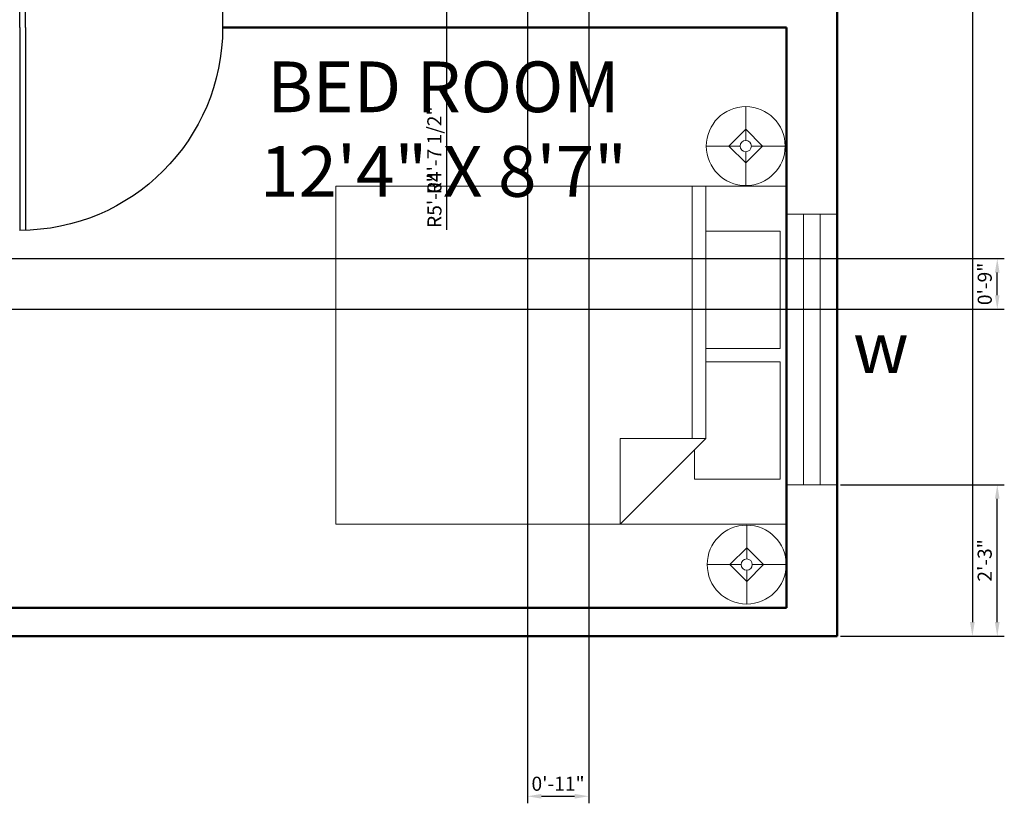
# Model space of a CAD drawing. Units: inches. Extents: x 1962 to 2423, y 2693 to 3296.
# Tile 2 of 4: x 2212 to 2386, y 2694 to 2833. Entities that reach past the tile are written whole.
import ezdxf

# ---------------------------------------------------------------- set-up
doc = ezdxf.new("R2010")
doc.units = ezdxf.units.IN
for name, color, linetype, lineweight in [('A-ANNO-DIMS', 2, 'Continuous', 18), ('A-ANNO-TEXT', 3, 'Continuous', 18), ('A-AREA-IDEN', 7, 'Continuous', 25), ('A-DOOR', 3, 'Continuous', 25), ('A-FURN', 8, 'Continuous', 18), ('A-GLAZ', 4, 'Continuous', 18), ('A-WALL', 7, 'Continuous', 50)]:
    doc.layers.add(name, color=color, linetype=linetype, lineweight=lineweight)
doc.styles.get("Standard").update_dxf_attribs({"font": 'arial.ttf'})
doc.dimstyles.new('ISO-25', dxfattribs={"dimtxt": 2.5, "dimasz": 2.5, "dimexe": 1.25, "dimexo": 0.625, "dimtad": 1, "dimdec": 0, "dimlunit": 3, "dimtxsty": 'Standard', "dimcen": 2.5, "dimadec": 0, "dimazin": 0, "dimtfac": 1, "dimtdec": 0, "dimtmove": 0, "dimatfit": 3, "dimfxl": 1, "dimarcsym": 0})

# ---------------------------------------------------------------- blocks, each defined once
blk = doc.blocks.new('*D13')
at = {"layer": 'A-ANNO-DIMS', "color": 0, "lineweight": -2, "transparency": 16777216}
for p, q in [((2357.16, 3263.59), (2381.77, 3263.59)), ((2380.52, 3261.09), (2380.52, 2726.09)), ((2357.16, 2723.59), (2381.77, 2723.59))]:
    blk.add_line(p, q, dxfattribs=at)
at = {"layer": 'A-ANNO-DIMS', "color": 0, "transparency": 16777216}
for points in [[(2380.1, 3261.09), (2380.94, 3261.09), (2380.52, 3263.59)], [(2380.1, 2726.09), (2380.94, 2726.09), (2380.52, 2723.59)]]:
    blk.add_solid(points, dxfattribs=at)
at = {"layer": 'Defpoints', "color": 0, "transparency": 16777216}
for p in [(2356.54, 3263.59), (2356.54, 2723.59), (2380.52, 2723.59)]:
    blk.add_point(p, dxfattribs=at)
at = {"layer": 'A-ANNO-DIMS', "color": 0, "transparency": 16777216, "insert": (2378.62, 2993.59), "char_height": 2.5, "attachment_point": 5, "rotation": 90}
blk.add_mtext("45'", dxfattribs=at)
blk = doc.blocks.new('Bed - Queen')
for p, q in [((0, -80.00003), (0, 0)), ((0, 0), (59.99999, 0)), ((59.99999, 0), (59.99999, -80.00003)), ((7.99999, -1.2), (28.79998, -1.2)), ((7.99999, -14.4), (7.99999, -1.2)), ((28.79998, -1.2), (28.79998, -14.4)), ((31.19999, -1.2), (51.99999, -1.2)), ((31.19999, -14.4), (31.19999, -1.2)), ((51.99999, -1.2), (51.99999, -16.4)), ((0, -14.4), (44.8, -14.4)), ((59.99999, -29.6), (44.8, -14.4)), ((44.8, -14.4), (44.8, -29.6)), ((44.8, -16.8), (0, -16.8)), ((51.99999, -16.4), (46.79936, -16.4)), ((44.8, -29.6), (59.99999, -29.6)), ((59.99999, -80.00003), (0, -80.00003))]:
    blk.add_line(p, q)
blk = doc.blocks.new('Lamp - Table')
for p, q in [((0, 7), (0, 1)), ((0, 3), (-3, 0)), ((3, 0), (0, 3)), ((-1, 0), (-7, 0)), ((-3, 0), (0, -3)), ((0, -3), (3, 0)), ((1, 0), (7, 0)), ((0, -1), (0, -7))]:
    blk.add_line(p, q)
for radius in [7, 1]:
    blk.add_circle((0, 0), radius)
blk = doc.blocks.new('DOOR-SWING-36IN')
for p, q in [((0, 5), (0, 41)), ((1, 5), (1, 41)), ((0, 5), (0, 0)), ((1, 5), (1, 0)), ((36, 0), (36, 5))]:
    blk.add_line(p, q)
blk.add_arc((0, 5), 36, 0, 90)
blk = doc.blocks.new('WINDOW-48IN')
for p, q in [((0, 48), (0, 0)), ((9, 48), (0, 48)), ((3, 48), (3, 0)), ((6, 0), (6, 48)), ((9, 0), (9, 48)), ((0, 0), (9, 0))]:
    blk.add_line(p, q)
blk = doc.blocks.new('*D62')
at = {"layer": 'A-ANNO-DIMS', "color": 0, "lineweight": -2, "transparency": 16777216}
for p, q in [((2357.16, 2750.46), (2386.19, 2750.46)), ((2384.94, 2726.09), (2384.94, 2747.96)), ((2357.16, 2723.59), (2386.19, 2723.59))]:
    blk.add_line(p, q, dxfattribs=at)
at = {"layer": 'A-ANNO-DIMS', "color": 0, "transparency": 16777216}
for points in [[(2384.52, 2747.96), (2385.35, 2747.96), (2384.94, 2750.46)], [(2384.52, 2726.09), (2385.35, 2726.09), (2384.94, 2723.59)]]:
    blk.add_solid(points, dxfattribs=at)
at = {"layer": 'Defpoints', "color": 0, "transparency": 16777216}
for p in [(2356.54, 2750.46), (2384.94, 2750.46), (2356.54, 2723.59)]:
    blk.add_point(p, dxfattribs=at)
at = {"layer": 'A-ANNO-DIMS', "color": 0, "transparency": 16777216, "insert": (2383.03, 2737.03), "char_height": 2.5, "attachment_point": 5, "rotation": 90}
blk.add_mtext('2\'-3"', dxfattribs=at)
blk = doc.blocks.new('*D65')
at = {"layer": 'A-ANNO-DIMS', "color": 0, "lineweight": -2, "transparency": 16777216}
for p, q in [((2301.59, 2881.95), (2301.59, 2693.94)), ((2312.47, 2879.27), (2312.47, 2693.94)), ((2304.09, 2695.19), (2309.97, 2695.19))]:
    blk.add_line(p, q, dxfattribs=at)
at = {"layer": 'A-ANNO-DIMS', "color": 0, "transparency": 16777216}
for points in [[(2304.09, 2695.61), (2304.09, 2694.77), (2301.59, 2695.19)], [(2309.97, 2695.61), (2309.97, 2694.77), (2312.47, 2695.19)]]:
    blk.add_solid(points, dxfattribs=at)
at = {"layer": 'Defpoints', "color": 0, "transparency": 16777216}
for p in [(2301.59, 2882.58), (2312.47, 2879.9), (2312.47, 2695.19)]:
    blk.add_point(p, dxfattribs=at)
at = {"layer": 'A-ANNO-DIMS', "color": 0, "transparency": 16777216, "insert": (2307.03, 2697.09), "char_height": 2.5, "attachment_point": 5}
blk.add_mtext('0\'-11"', dxfattribs=at)
blk = doc.blocks.new('*D69')
at = {"layer": 'A-ANNO-DIMS', "color": 0, "lineweight": -2, "transparency": 16777216}
for p, q in [((2042.16, 2790.59), (2386.19, 2790.59)), ((2384.94, 2784.09), (2384.94, 2788.09)), ((2042.16, 2781.59), (2386.19, 2781.59))]:
    blk.add_line(p, q, dxfattribs=at)
at = {"layer": 'A-ANNO-DIMS', "color": 0, "transparency": 16777216}
for points in [[(2384.52, 2788.09), (2385.35, 2788.09), (2384.94, 2790.59)], [(2384.52, 2784.09), (2385.35, 2784.09), (2384.94, 2781.59)]]:
    blk.add_solid(points, dxfattribs=at)
at = {"layer": 'Defpoints', "color": 0, "transparency": 16777216}
for p in [(2041.54, 2790.59), (2384.94, 2790.59), (2041.54, 2781.59)]:
    blk.add_point(p, dxfattribs=at)
at = {"layer": 'A-ANNO-DIMS', "color": 0, "transparency": 16777216, "insert": (2383.04, 2786.09), "char_height": 2.5, "attachment_point": 5, "rotation": 90}
blk.add_mtext('0\'-9"', dxfattribs=at)
blk = doc.blocks.new('*D74')
at = {"layer": 'A-ANNO-DIMS', "color": 0, "lineweight": -2, "transparency": 16777216}
for p, q in [((2287.33, 2897.26), (2287.33, 2837.01)), ((2287.33, 2795.71), (2287.33, 2834.51))]:
    blk.add_line(p, q, dxfattribs=at)
at = {"layer": 'A-ANNO-DIMS', "color": 0, "transparency": 16777216}
blk.add_solid([(2286.91, 2834.51), (2287.74, 2834.51), (2287.33, 2837.01)], dxfattribs=at)
at = {"layer": 'Defpoints', "color": 0, "transparency": 16777216}
for p in [(2287.33, 2897.26), (2287.33, 2837.01)]:
    blk.add_point(p, dxfattribs=at)
at = {"layer": 'A-ANNO-DIMS', "color": 0, "transparency": 16777216, "insert": (2285.43, 2800.86), "char_height": 2.5, "attachment_point": 5, "rotation": 89.9997}
blk.add_mtext('R5\'-0"', dxfattribs=at)
blk = doc.blocks.new('*D75')
at = {"layer": 'A-ANNO-DIMS', "color": 0, "lineweight": -2, "transparency": 16777216}
for p, q in [((2287.33, 2898.39), (2287.33, 2843.01)), ((2287.33, 2801.72), (2287.33, 2840.51))]:
    blk.add_line(p, q, dxfattribs=at)
at = {"layer": 'A-ANNO-DIMS', "color": 0, "transparency": 16777216}
blk.add_solid([(2286.91, 2840.51), (2287.74, 2840.51), (2287.33, 2843.01)], dxfattribs=at)
at = {"layer": 'Defpoints', "color": 0, "transparency": 16777216}
for p in [(2287.33, 2898.39), (2287.33, 2843.01)]:
    blk.add_point(p, dxfattribs=at)
at = {"layer": 'A-ANNO-DIMS', "color": 0, "transparency": 16777216, "insert": (2285.41, 2809.78), "char_height": 2.5, "attachment_point": 5, "rotation": 89.9996}
blk.add_mtext('R4\'-7 1/2"', dxfattribs=at)

msp = doc.modelspace()

# ---------------------------------------------------------------- linework, layer by layer
at = {"layer": 'A-WALL'}
for p, q in [((2356.54, 2723.59), (2356.54, 3263.59)), ((2247.54, 2831.59), (2347.54, 2831.59)), ((2347.54, 2728.59), (2347.54, 2831.59)), ((2199.54, 2728.59), (2347.54, 2728.59)), ((1996.54, 2723.59), (2356.54, 2723.59))]:
    msp.add_line(p, q, dxfattribs=at)

# ---------------------------------------------------------------- block references
at = {"layer": 'A-DOOR', "extrusion": (0, 0, -1), "zscale": -1, "rotation": 180}
msp.add_blockref('DOOR-SWING-36IN', (-2211.54, 2836.59), dxfattribs=at)
at = {"layer": 'A-FURN', "rotation": 270}
for name, p in [('Lamp - Table', (2340.32, 2810.54)), ('Bed - Queen', (2347.63, 2803.44)), ('Lamp - Table', (2340.49, 2736.29))]:
    msp.add_blockref(name, p, dxfattribs=at)
at = {"layer": 'A-GLAZ'}
msp.add_blockref('WINDOW-48IN', (2347.54, 2750.46), dxfattribs=at)

# ---------------------------------------------------------------- texts
at = {"layer": 'A-ANNO-TEXT', "insert": (2353.54, 2779.27), "char_height": 9, "attachment_point": 1}
msp.add_mtext_dynamic_manual_height_columns('\\pxqc;w', width=21.5056, gutter_width=12.5, heights=[0], dxfattribs=at)
at = {"layer": 'A-AREA-IDEN', "insert": (2235.77, 2825.55), "char_height": 9, "attachment_point": 1}
msp.add_mtext_dynamic_manual_height_columns('\\pxqc;BED ROOM \\P12\'4" X 8\'7"', width=101.8726, gutter_width=12.5, heights=[0], dxfattribs=at)

# ---------------------------------------------------------------- dimensions: what is measured, and where the dimension line sits
at = {"layer": 'A-ANNO-DIMS'}
for base, p1, p2, override, picture, middle in [((2380.52, 2723.59), (2356.54, 3263.59), (2356.54, 2723.59), {"dimclrd": 0, "dimclre": 0, "dimclrt": 0}, '*D13', (2378.62, 2993.59)), ((2384.94, 2790.59), (2041.54, 2781.59), (2041.54, 2790.59), {"dimdec": 1, "dimlfac": 1, "dimrnd": 0, "dimzin": 1, "dimdsep": 46, "dimlunit": 4, "dimfrac": 2}, '*D69', (2383.04, 2786.09)), ((2384.94, 2750.46), (2356.54, 2723.59), (2356.54, 2750.46), {"dimdec": 1, "dimlfac": 1, "dimrnd": 0, "dimzin": 1, "dimdsep": 46, "dimlunit": 4, "dimfrac": 2}, '*D62', (2383.03, 2737.03))]:
    dim = msp.add_linear_dim(base=base, p1=p1, p2=p2, angle=90, dimstyle='ISO-25', override=override, dxfattribs=at)
    dim.commit()
    dim.dimension.update_dxf_attribs({"geometry": picture, "text_midpoint": middle})
for center, mpoint, picture, middle in [((2287.33, 2898.39), (2287.33, 2843.01), '*D75', (2287.33, 2809.78)), ((2287.32836, 2897.25625), (2287.328, 2837.00627), '*D74', (2287.32779, 2800.85628))]:
    dim = msp.add_radius_dim(center=center, mpoint=mpoint, dimstyle='ISO-25', override={"dimdec": 1, "dimlfac": 1, "dimrnd": 0, "dimzin": 1, "dimdsep": 46, "dimlunit": 4, "dimfrac": 2}, dxfattribs=at)
    dim.commit()
    dim.dimension.update_dxf_attribs({"geometry": picture, "text_midpoint": middle, "dimtype": 164})
dim = msp.add_linear_dim(base=(2312.47, 2695.19), p1=(2301.59, 2882.58), p2=(2312.47, 2879.9), dimstyle='ISO-25', override={"dimdec": 1, "dimlfac": 1, "dimrnd": 0, "dimzin": 1, "dimdsep": 46, "dimlunit": 4, "dimfrac": 2}, dxfattribs=at)
dim.commit()
dim.dimension.update_dxf_attribs({"geometry": '*D65', "text_midpoint": (2307.03, 2697.09)})

doc.saveas('drawing.dxf')
